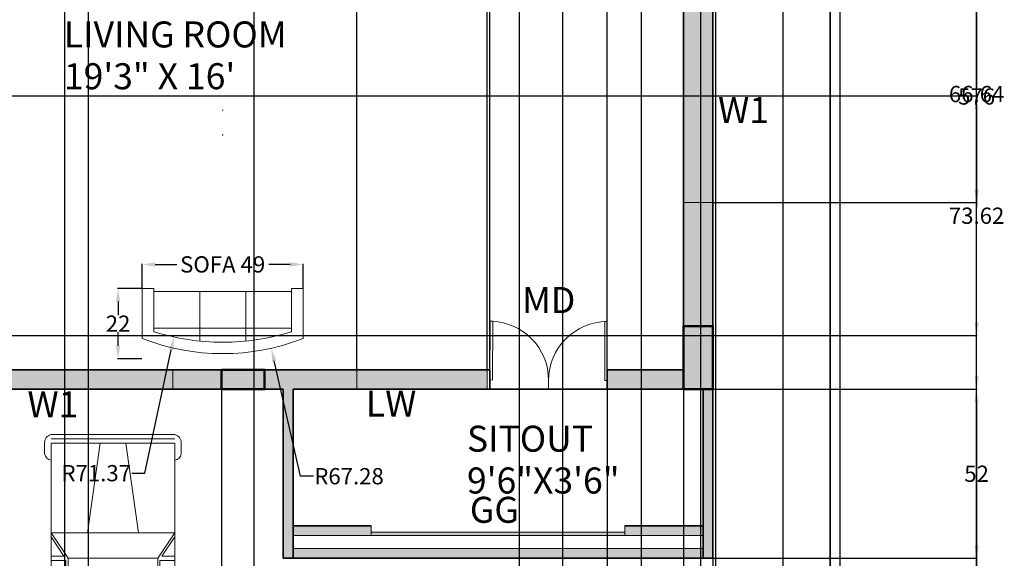
# Model space of a CAD drawing. Units: inches. Extents: x 460 to 1030, y -658 to 271.
# Tile 6 of 10: x 728 to 1030, y -340 to -174. Entities that reach past the tile are written whole.
import ezdxf

# ---------------------------------------------------------------- set-up
doc = ezdxf.new("R2010")
doc.units = ezdxf.units.IN
doc.header["$MEASUREMENT"] = 0
for name, color, linetype, lineweight in [('A-ANNO-DIMS', 2, 'Continuous', 18), ('A-ANNO-TEXT', 7, 'Continuous', 18), ('A-AREA-IDEN', 7, 'Continuous', 25), ('A-COLS', 7, 'Continuous', 50), ('A-DOOR', 3, 'Continuous', 20), ('A-FLOR-STRS', 7, 'Continuous', 18), ('A-FURN', 8, 'Continuous', 18), ('A-GLAZ', 4, 'Continuous', 20), ('A-GLAZ-PATT', 4, 'Continuous', 13), ('A-WALL', 7, 'Continuous', 35), ('A-WALL-PATT', 5, 'Continuous', 13), ('C-PROP', 7, 'Continuous', 25), ('C-SITE-VEHI', 8, 'Continuous', 13)]:
    doc.layers.add(name, color=color, linetype=linetype, lineweight=lineweight)
doc.layers.add('A-COLS-PATT', color=7, linetype='Continuous', lineweight=13, true_color=0xffffff)
doc.styles.get("Standard").update_dxf_attribs({"font": 'arial.ttf'})
doc.dimstyles.get("Standard").update_dxf_attribs({"dimtxt": 5, "dimasz": 4, "dimexe": 0.18, "dimexo": 0.0625, "dimgap": 0.09, "dimtad": 0, "dimtih": 1, "dimtoh": 1, "dimdec": 1, "dimzin": 0, "dimdsep": 46, "dimlunit": 4, "dimtxsty": 'Standard', "dimcen": 0.09, "dimadec": 0, "dimazin": 0, "dimtfac": 1, "dimtdec": 1, "dimtofl": 0, "dimtmove": 0, "dimatfit": 3, "dimfxl": 1, "dimtolj": 1, "dimtzin": 0, "dimarcsym": 0})

# ---------------------------------------------------------------- blocks, each defined once
blk = doc.blocks.new('*U2')
for p, q in [((0, 0), (0, -6)), ((40, 0), (40, -6))]:
    blk.add_line(p, q)
blk.add_lwpolyline([(0, 0), (0, 40), (1.75, 40), (1.75, 0)], close=True)
blk.add_arc((0, 0), 40, 0, 90)
blk = doc.blocks.new('Sofa - Roundback 7 ft.')
for p, q in [((-12.00002, -32.4421), (-12.00003, -6.5971)), ((11.99997, -32.4421), (11.99998, -6.5971)), ((-36.000027, -34), (-36.000027, -11.4696)), ((-35.999844, -13.3819), (35.9998, -13.3819)), ((35.99998, -34), (35.99998, -11.4696)), ((-36.000027, -32.4421), (35.99998, -32.4421))]:
    blk.add_line(p, q)
for points in [[(-36.000027, -34), (-42.000027, -34), (-42.000027, -8)], [(41.99998, -8), (41.99998, -34), (35.99998, -34)]]:
    blk.add_lwpolyline(points)
for centre, radius, start, end in [((0, -114.25), 114.25, 68.43141, 111.5686), ((-0.00001, -127.1968), 121.1968, 72.72033, 107.2797)]:
    blk.add_arc(centre, radius, start, end)
blk = doc.blocks.new('*U14')
for p, q in [((3, -10), (3, 974)), ((70, -10), (70, 973)), ((138, 1075), (308, 1075)), ((138, 973), (410, 973)), ((138, -10), (138, 971)), ((410, 973), (4581, 973)), ((1563, -10), (1563, 973)), ((1563, 973), (1969, 702)), ((1630, 973), (1936, 769)), ((1936, 769), (1936, 973)), ((2003, 973), (2003, 736)), ((2716, 736), (2716, 973)), ((2783, 702), (2783, 973)), ((2851, 973), (2851, 736)), ((3563, 736), (3563, 973)), ((3597, 702), (3801, 973)), ((3801, -10), (3801, 973)), ((4818, 973), (4547, 973)), ((4818, 1075), (4649, 1075)), ((4818, -10), (4818, 971)), ((4886, -10), (4886, 973)), ((4954, -10), (4954, 974)), ((1969, 702), (3597, 702)), ((1969, -10), (1969, 702)), ((2003, 736), (2716, 736)), ((2851, 736), (3563, 736)), ((3597, -10), (3597, 702)), ((138, 193), (1563, 396)), ((3, -11), (3, -995)), ((70, -10), (70, -994)), ((138, -11), (138, -992)), ((1563, -10), (1563, -994)), ((1969, -10), (1969, -723)), ((3597, -10), (3597, -723)), ((3801, -10), (3801, -994)), ((4818, -11), (4818, -992)), ((4886, -10), (4886, -994)), ((4954, -11), (4954, -995)), ((138, -214), (1563, -417)), ((1563, -994), (1969, -723)), ((1969, -723), (3597, -723)), ((2003, -994), (2003, -757)), ((2003, -757), (2716, -757)), ((2716, -757), (2716, -994)), ((2783, -723), (2783, -994)), ((2851, -757), (3563, -757)), ((2851, -994), (2851, -757)), ((3563, -757), (3563, -994)), ((3597, -723), (3801, -994)), ((1630, -994), (1936, -790)), ((1936, -790), (1936, -994)), ((138, -994), (410, -994)), ((138, -1096), (308, -1096)), ((410, -994), (4581, -994)), ((4818, -994), (4547, -994)), ((4818, -1096), (4649, -1096))]:
    blk.add_line(p, q)
for centre, radius, start, end in [((128, 946), 129, 85.6455, 168.0943), ((291, 956), 120, 8.1301, 81.87), ((4665, 956), 120, 98.13, 171.8699), ((4828, 946), 129, 11.9057, 94.3545), ((128, -967), 129, 191.9057, 274.3545), ((291, -977), 120, 278.13, 351.8699), ((4665, -977), 120, 188.1301, 261.87), ((4828, -967), 129, 265.6455, 348.0943)]:
    blk.add_arc(centre, radius, start, end)
blk = doc.blocks.new('*D37')
at = {"layer": 'A-ANNO-DIMS', "color": 0, "lineweight": -2, "transparency": 16777216}
for p, q in [((765.43, -256.72), (765.43, -249.18)), ((769.43, -249.36), (776.02, -249.36)), ((810.89, -249.36), (804.3, -249.36)), ((814.89, -256.72), (814.89, -249.18))]:
    blk.add_line(p, q, dxfattribs=at)
at = {"layer": 'A-ANNO-DIMS', "color": 0, "transparency": 16777216}
for points in [[(769.43, -248.7), (769.43, -250.03), (765.43, -249.36)], [(810.89, -248.7), (810.89, -250.03), (814.89, -249.36)]]:
    blk.add_solid(points, dxfattribs=at)
at = {"layer": 'Defpoints', "color": 0, "transparency": 16777216}
for p in [(765.43, -249.36), (765.43, -256.78), (814.89, -256.78)]:
    blk.add_point(p, dxfattribs=at)
at = {"layer": 'A-ANNO-DIMS', "color": 0, "transparency": 16777216, "insert": (790.16, -249.36), "char_height": 5, "attachment_point": 5}
blk.add_mtext('\\A1;SOFA 49', dxfattribs=at)
blk = doc.blocks.new('*D38')
at = {"layer": 'A-ANNO-DIMS', "color": 0, "lineweight": -2, "transparency": 16777216}
for p, q in [((765.36, -256.78), (757.83, -256.78)), ((758.01, -260.78), (758.01, -264.98)), ((758.01, -274.37), (758.01, -270.18)), ((765.36, -278.37), (757.83, -278.37))]:
    blk.add_line(p, q, dxfattribs=at)
at = {"layer": 'A-ANNO-DIMS', "color": 0, "transparency": 16777216}
for points in [[(757.34, -260.78), (758.67, -260.78), (758.01, -256.78)], [(757.34, -274.37), (758.67, -274.37), (758.01, -278.37)]]:
    blk.add_solid(points, dxfattribs=at)
at = {"layer": 'Defpoints', "color": 0, "transparency": 16777216}
for p in [(765.43, -256.78), (758.01, -278.37), (765.43, -278.37)]:
    blk.add_point(p, dxfattribs=at)
at = {"layer": 'A-ANNO-DIMS', "color": 0, "transparency": 16777216, "insert": (758.01, -267.58), "char_height": 5, "attachment_point": 5}
blk.add_mtext('\\A1;22', dxfattribs=at)
blk = doc.blocks.new('*D41')
at = {"layer": 'A-ANNO-DIMS', "color": 0, "lineweight": -2, "transparency": 16777216}
for p, q in [((979.86, 129.27), (1022.03, 129.27)), ((1021.85, 125.27), (1021.85, -76.63)), ((1021.85, -283.73), (1021.85, -81.83)), ((940.86, -287.73), (1022.03, -287.73))]:
    blk.add_line(p, q, dxfattribs=at)
at = {"layer": 'A-ANNO-DIMS', "color": 0, "transparency": 16777216}
for points in [[(1021.18, 125.27), (1022.51, 125.27), (1021.85, 129.27)], [(1021.18, -283.73), (1022.51, -283.73), (1021.85, -287.73)]]:
    blk.add_solid(points, dxfattribs=at)
at = {"layer": 'Defpoints', "color": 0, "transparency": 16777216}
for p in [(979.8, 129.27), (1021.85, 129.27), (940.8, -287.73)]:
    blk.add_point(p, dxfattribs=at)
at = {"layer": 'A-ANNO-DIMS', "color": 0, "transparency": 16777216, "insert": (1021.85, -79.23), "char_height": 5, "attachment_point": 5}
blk.add_mtext('\\A1;417', dxfattribs=at)
blk = doc.blocks.new('*D42')
at = {"layer": 'A-ANNO-DIMS', "color": 0, "lineweight": -2, "transparency": 16777216}
for p, q in [((940.86, -287.73), (1022.03, -287.73)), ((1021.85, -291.73), (1021.85, -447.08)), ((1021.85, -607.73), (1021.85, -452.37)), ((979.86, -611.73), (1022.03, -611.73))]:
    blk.add_line(p, q, dxfattribs=at)
at = {"layer": 'A-ANNO-DIMS', "color": 0, "transparency": 16777216}
for points in [[(1021.18, -291.73), (1022.51, -291.73), (1021.85, -287.73)], [(1021.18, -607.73), (1022.51, -607.73), (1021.85, -611.73)]]:
    blk.add_solid(points, dxfattribs=at)
at = {"layer": 'Defpoints', "color": 0, "transparency": 16777216}
for p in [(940.8, -287.73), (1021.85, -287.73), (979.8, -611.73)]:
    blk.add_point(p, dxfattribs=at)
at = {"layer": 'A-ANNO-DIMS', "color": 0, "transparency": 16777216, "insert": (1021.85, -449.73), "char_height": 5, "attachment_point": 5}
blk.add_mtext('\\A1;324', dxfattribs=at)
blk = doc.blocks.new('*D44')
at = {"layer": 'A-ANNO-DIMS', "color": 0, "lineweight": -2, "transparency": 16777216}
for p, q in [((940.86, 90.27), (1022.03, 90.27)), ((1021.85, 86.27), (1021.85, -195.08)), ((1021.85, -481.73), (1021.85, -200.37)), ((979.86, -485.73), (1022.03, -485.73))]:
    blk.add_line(p, q, dxfattribs=at)
at = {"layer": 'A-ANNO-DIMS', "color": 0, "transparency": 16777216}
for points in [[(1021.18, 86.27), (1022.51, 86.27), (1021.85, 90.27)], [(1021.18, -481.73), (1022.51, -481.73), (1021.85, -485.73)]]:
    blk.add_solid(points, dxfattribs=at)
at = {"layer": 'Defpoints', "color": 0, "transparency": 16777216}
for p in [(940.8, 90.27), (979.8, -485.73), (1021.85, -485.73)]:
    blk.add_point(p, dxfattribs=at)
at = {"layer": 'A-ANNO-DIMS', "color": 0, "transparency": 16777216, "insert": (1021.85, -197.73), "char_height": 5, "attachment_point": 5}
blk.add_mtext('\\A1;576', dxfattribs=at)
blk = doc.blocks.new('*D45')
at = {"layer": 'A-ANNO-DIMS', "color": 0, "lineweight": -2, "transparency": 16777216}
for p, q in [((976.8, 126.21), (976.8, -654.61)), ((940.8, 90.21), (940.8, -654.61)), ((944.8, -654.43), (955.13, -654.43)), ((972.8, -654.43), (962.46, -654.43))]:
    blk.add_line(p, q, dxfattribs=at)
at = {"layer": 'A-ANNO-DIMS', "color": 0, "transparency": 16777216}
for points in [[(944.8, -653.77), (944.8, -655.1), (940.8, -654.43)], [(972.8, -653.77), (972.8, -655.1), (976.8, -654.43)]]:
    blk.add_solid(points, dxfattribs=at)
at = {"layer": 'Defpoints', "color": 0, "transparency": 16777216}
for p in [(976.8, 126.27), (940.8, 90.27), (976.8, -654.43)]:
    blk.add_point(p, dxfattribs=at)
at = {"layer": 'A-ANNO-DIMS', "color": 0, "transparency": 16777216, "insert": (958.8, -654.43), "char_height": 5, "attachment_point": 5}
blk.add_mtext('\\A1;36', dxfattribs=at)
blk = doc.blocks.new('*D46')
at = {"layer": 'A-ANNO-DIMS', "color": 0, "lineweight": -2, "transparency": 16777216}
for p, q in [((936.98, 127.21), (936.98, -654.61)), ((962.32, 127.21), (962.32, -654.61)), ((932.98, -654.43), (928.98, -654.43)), ((966.32, -654.43), (970.32, -654.43))]:
    blk.add_line(p, q, dxfattribs=at)
at = {"layer": 'A-ANNO-DIMS', "color": 0, "transparency": 16777216}
for points in [[(932.98, -653.77), (932.98, -655.1), (936.98, -654.43)], [(966.32, -653.77), (966.32, -655.1), (962.32, -654.43)]]:
    blk.add_solid(points, dxfattribs=at)
at = {"layer": 'Defpoints', "color": 0, "transparency": 16777216}
for p in [(936.98, 127.27), (962.32, 127.27), (962.32, -654.43)]:
    blk.add_point(p, dxfattribs=at)
at = {"layer": 'A-ANNO-DIMS', "color": 0, "transparency": 16777216, "insert": (949.65, -654.43), "char_height": 5, "attachment_point": 5}
blk.add_mtext('\\A1;25.346', dxfattribs=at)
blk = doc.blocks.new('*D47')
at = {"layer": 'A-ANNO-DIMS', "color": 0, "lineweight": -2, "transparency": 16777216}
for p, q in [((962.32, 129.21), (962.32, -654.61)), ((979.8, 129.21), (979.8, -654.61)), ((966.32, -654.43), (975.8, -654.43)), ((979.8, -654.43), (983.8, -654.43))]:
    blk.add_line(p, q, dxfattribs=at)
at = {"layer": 'A-ANNO-DIMS', "color": 0, "transparency": 16777216}
for points in [[(966.32, -653.77), (966.32, -655.1), (962.32, -654.43)], [(975.8, -653.77), (975.8, -655.1), (979.8, -654.43)]]:
    blk.add_solid(points, dxfattribs=at)
at = {"layer": 'Defpoints', "color": 0, "transparency": 16777216}
for p in [(962.32, 129.27), (979.8, 129.27), (979.8, -654.43)]:
    blk.add_point(p, dxfattribs=at)
at = {"layer": 'A-ANNO-DIMS', "color": 0, "transparency": 16777216, "insert": (994.02, -654.43), "char_height": 5, "attachment_point": 5}
blk.add_mtext('\\A1;17.474', dxfattribs=at)
blk = doc.blocks.new('*D48')
at = {"layer": 'A-ANNO-DIMS', "color": 0, "lineweight": -2, "transparency": 16777216}
for p, q in [((799.88, -611.66), (799.88, 267.89)), ((803.88, 267.71), (860.58, 267.71)), ((937.7, 267.71), (881, 267.71)), ((941.7, -611.66), (941.7, 267.89))]:
    blk.add_line(p, q, dxfattribs=at)
at = {"layer": 'A-ANNO-DIMS', "color": 0, "transparency": 16777216}
for points in [[(803.88, 268.38), (803.88, 267.04), (799.88, 267.71)], [(937.7, 268.38), (937.7, 267.04), (941.7, 267.71)]]:
    blk.add_solid(points, dxfattribs=at)
at = {"layer": 'Defpoints', "color": 0, "transparency": 16777216}
for p in [(941.7, 267.71), (799.88, -611.73), (941.7, -611.73)]:
    blk.add_point(p, dxfattribs=at)
at = {"layer": 'A-ANNO-DIMS', "color": 0, "transparency": 16777216, "insert": (870.79, 267.71), "char_height": 5, "attachment_point": 5}
blk.add_mtext('\\A1;141.82', dxfattribs=at)
blk = doc.blocks.new('*D49')
at = {"layer": 'A-ANNO-DIMS', "color": 0, "lineweight": -2, "transparency": 16777216}
for p, q in [((941.7, -608.66), (941.7, 267.89)), ((945.7, 267.71), (953.15, 267.71)), ((972.8, 267.71), (965.35, 267.71)), ((976.8, -608.66), (976.8, 267.89))]:
    blk.add_line(p, q, dxfattribs=at)
at = {"layer": 'A-ANNO-DIMS', "color": 0, "transparency": 16777216}
for points in [[(945.7, 268.38), (945.7, 267.04), (941.7, 267.71)], [(972.8, 268.38), (972.8, 267.04), (976.8, 267.71)]]:
    blk.add_solid(points, dxfattribs=at)
at = {"layer": 'Defpoints', "color": 0, "transparency": 16777216}
for p in [(976.8, 267.71), (941.7, -608.73), (976.8, -608.73)]:
    blk.add_point(p, dxfattribs=at)
at = {"layer": 'A-ANNO-DIMS', "color": 0, "transparency": 16777216, "insert": (959.25, 267.71), "char_height": 5, "attachment_point": 5}
blk.add_mtext('\\A1;35.1', dxfattribs=at)
blk = doc.blocks.new('*D52')
at = {"layer": 'A-ANNO-DIMS', "color": 0, "lineweight": -2, "transparency": 16777216}
for p, q in [((872.3, -281.66), (872.3, 267.89)), ((876.3, 267.71), (879.84, 267.71)), ((904.35, 267.71), (900.81, 267.71)), ((908.35, -281.66), (908.35, 267.89))]:
    blk.add_line(p, q, dxfattribs=at)
at = {"layer": 'A-ANNO-DIMS', "color": 0, "transparency": 16777216}
for points in [[(876.3, 268.38), (876.3, 267.04), (872.3, 267.71)], [(904.35, 268.38), (904.35, 267.04), (908.35, 267.71)]]:
    blk.add_solid(points, dxfattribs=at)
at = {"layer": 'Defpoints', "color": 0, "transparency": 16777216}
for p in [(908.35, 267.71), (872.3, -281.73), (908.35, -281.73)]:
    blk.add_point(p, dxfattribs=at)
at = {"layer": 'A-ANNO-DIMS', "color": 0, "transparency": 16777216, "insert": (890.32, 267.71), "char_height": 5, "attachment_point": 5}
blk.add_mtext('\\A1;36.045', dxfattribs=at)
blk = doc.blocks.new('*D53')
at = {"layer": 'A-ANNO-DIMS', "color": 0, "lineweight": -2, "transparency": 16777216}
for p, q in [((908.35, -281.79), (908.35, -654.61)), ((931.8, -281.79), (931.8, -654.61)), ((904.35, -654.43), (900.35, -654.43)), ((935.8, -654.43), (939.8, -654.43))]:
    blk.add_line(p, q, dxfattribs=at)
at = {"layer": 'A-ANNO-DIMS', "color": 0, "transparency": 16777216}
for points in [[(904.35, -653.77), (904.35, -655.1), (908.35, -654.43)], [(935.8, -653.77), (935.8, -655.1), (931.8, -654.43)]]:
    blk.add_solid(points, dxfattribs=at)
at = {"layer": 'Defpoints', "color": 0, "transparency": 16777216}
for p in [(908.35, -281.73), (931.8, -281.73), (931.8, -654.43)]:
    blk.add_point(p, dxfattribs=at)
at = {"layer": 'A-ANNO-DIMS', "color": 0, "transparency": 16777216, "insert": (920.07, -654.43), "char_height": 5, "attachment_point": 5}
blk.add_mtext('\\A1;23.45', dxfattribs=at)
blk = doc.blocks.new('*D54')
at = {"layer": 'A-ANNO-DIMS', "color": 0, "lineweight": -2, "transparency": 16777216}
for p, q in [((894.61, -141.78), (894.61, -654.61)), ((931.8, -141.78), (931.8, -654.61)), ((898.61, -654.43), (904.68, -654.43)), ((927.8, -654.43), (921.73, -654.43))]:
    blk.add_line(p, q, dxfattribs=at)
at = {"layer": 'A-ANNO-DIMS', "color": 0, "transparency": 16777216}
for points in [[(898.61, -653.77), (898.61, -655.1), (894.61, -654.43)], [(927.8, -653.77), (927.8, -655.1), (931.8, -654.43)]]:
    blk.add_solid(points, dxfattribs=at)
at = {"layer": 'Defpoints', "color": 0, "transparency": 16777216}
for p in [(894.61, -141.72), (931.8, -141.72), (931.8, -654.43)]:
    blk.add_point(p, dxfattribs=at)
at = {"layer": 'A-ANNO-DIMS', "color": 0, "transparency": 16777216, "insert": (913.2, -654.43), "char_height": 5, "attachment_point": 5}
blk.add_mtext('\\A1;37.18', dxfattribs=at)
blk = doc.blocks.new('*D57')
at = {"layer": 'A-ANNO-DIMS', "color": 0, "lineweight": -2, "transparency": 16777216}
for p, q in [((717.53, -38.79), (717.53, -654.61)), ((741.59, -38.79), (741.59, -654.61)), ((713.53, -654.43), (709.53, -654.43)), ((745.59, -654.43), (749.59, -654.43))]:
    blk.add_line(p, q, dxfattribs=at)
at = {"layer": 'A-ANNO-DIMS', "color": 0, "transparency": 16777216}
for points in [[(713.53, -653.77), (713.53, -655.1), (717.53, -654.43)], [(745.59, -653.77), (745.59, -655.1), (741.59, -654.43)]]:
    blk.add_solid(points, dxfattribs=at)
at = {"layer": 'Defpoints', "color": 0, "transparency": 16777216}
for p in [(717.53, -38.73), (741.59, -38.73), (741.59, -654.43)]:
    blk.add_point(p, dxfattribs=at)
at = {"layer": 'A-ANNO-DIMS', "color": 0, "transparency": 16777216, "insert": (729.56, -654.43), "char_height": 5, "attachment_point": 5}
blk.add_mtext('\\A1;24.065', dxfattribs=at)
blk = doc.blocks.new('*D60')
at = {"layer": 'A-ANNO-DIMS', "color": 0, "lineweight": -2, "transparency": 16777216}
for p, q in [((940.86, -163.66), (1022.03, -163.66)), ((1021.85, -167.66), (1021.85, -194.33)), ((1021.85, -226.29), (1021.85, -199.62)), ((940.86, -230.29), (1022.03, -230.29))]:
    blk.add_line(p, q, dxfattribs=at)
at = {"layer": 'A-ANNO-DIMS', "color": 0, "transparency": 16777216}
for points in [[(1021.18, -167.66), (1022.51, -167.66), (1021.85, -163.66)], [(1021.18, -226.29), (1022.51, -226.29), (1021.85, -230.29)]]:
    blk.add_solid(points, dxfattribs=at)
at = {"layer": 'Defpoints', "color": 0, "transparency": 16777216}
for p in [(940.8, -163.66), (940.8, -230.29), (1021.85, -230.29)]:
    blk.add_point(p, dxfattribs=at)
at = {"layer": 'A-ANNO-DIMS', "color": 0, "transparency": 16777216, "insert": (1021.85, -196.98), "char_height": 5, "attachment_point": 5}
blk.add_mtext('\\A1;66.64', dxfattribs=at)
blk = doc.blocks.new('*D62')
at = {"layer": 'A-ANNO-DIMS', "color": 0, "lineweight": -2, "transparency": 16777216}
for p, q in [((700.86, -197.58), (1022.03, -197.58)), ((1021.85, -201.58), (1021.85, -231.74)), ((1021.85, -267.2), (1021.85, -237.03)), ((700.86, -271.2), (1022.03, -271.2))]:
    blk.add_line(p, q, dxfattribs=at)
at = {"layer": 'A-ANNO-DIMS', "color": 0, "transparency": 16777216}
for points in [[(1021.18, -201.58), (1022.51, -201.58), (1021.85, -197.58)], [(1021.18, -267.2), (1022.51, -267.2), (1021.85, -271.2)]]:
    blk.add_solid(points, dxfattribs=at)
at = {"layer": 'Defpoints', "color": 0, "transparency": 16777216}
for p in [(700.8, -197.58), (700.8, -271.2), (1021.85, -271.2)]:
    blk.add_point(p, dxfattribs=at)
at = {"layer": 'A-ANNO-DIMS', "color": 0, "transparency": 16777216, "insert": (1021.85, -234.39), "char_height": 5, "attachment_point": 5}
blk.add_mtext('\\A1;73.62', dxfattribs=at)
blk = doc.blocks.new('*D67')
at = {"layer": 'A-ANNO-DIMS', "color": 0, "lineweight": -2, "transparency": 16777216}
for p, q in [((940.86, -287.73), (1022.03, -287.73)), ((1021.85, -291.73), (1021.85, -311.08)), ((1021.85, -335.73), (1021.85, -316.37)), ((940.86, -339.73), (1022.03, -339.73))]:
    blk.add_line(p, q, dxfattribs=at)
at = {"layer": 'A-ANNO-DIMS', "color": 0, "transparency": 16777216}
for points in [[(1021.18, -291.73), (1022.51, -291.73), (1021.85, -287.73)], [(1021.18, -335.73), (1022.51, -335.73), (1021.85, -339.73)]]:
    blk.add_solid(points, dxfattribs=at)
at = {"layer": 'Defpoints', "color": 0, "transparency": 16777216}
for p in [(940.8, -287.73), (1021.85, -287.73), (940.8, -339.73)]:
    blk.add_point(p, dxfattribs=at)
at = {"layer": 'A-ANNO-DIMS', "color": 0, "transparency": 16777216, "insert": (1021.85, -313.73), "char_height": 5, "attachment_point": 5}
blk.add_mtext('\\A1;52', dxfattribs=at)
blk = doc.blocks.new('*D69')
at = {"layer": 'A-ANNO-DIMS', "color": 0, "lineweight": -2, "transparency": 16777216}
for p, q in [((881.27, 90.21), (881.27, -654.61)), ((918.77, 90.21), (918.77, -654.61)), ((885.27, -654.43), (893.42, -654.43)), ((914.77, -654.43), (906.62, -654.43))]:
    blk.add_line(p, q, dxfattribs=at)
at = {"layer": 'A-ANNO-DIMS', "color": 0, "transparency": 16777216}
for points in [[(885.27, -653.77), (885.27, -655.1), (881.27, -654.43)], [(914.77, -653.77), (914.77, -655.1), (918.77, -654.43)]]:
    blk.add_solid(points, dxfattribs=at)
at = {"layer": 'Defpoints', "color": 0, "transparency": 16777216}
for p in [(881.27, 90.27), (918.77, 90.27), (918.77, -654.43)]:
    blk.add_point(p, dxfattribs=at)
at = {"layer": 'A-ANNO-DIMS', "color": 0, "transparency": 16777216, "insert": (900.02, -654.43), "char_height": 5, "attachment_point": 5}
blk.add_mtext('\\A1;37.5', dxfattribs=at)
blk = doc.blocks.new('*D70')
at = {"layer": 'A-ANNO-DIMS', "color": 0, "lineweight": -2, "transparency": 16777216}
for p, q in [((716.71, -287.79), (716.71, -654.61)), ((789.82, -287.79), (789.82, -654.61)), ((720.71, -654.43), (744.79, -654.43)), ((785.82, -654.43), (761.75, -654.43))]:
    blk.add_line(p, q, dxfattribs=at)
at = {"layer": 'A-ANNO-DIMS', "color": 0, "transparency": 16777216}
for points in [[(720.71, -653.77), (720.71, -655.1), (716.71, -654.43)], [(785.82, -653.77), (785.82, -655.1), (789.82, -654.43)]]:
    blk.add_solid(points, dxfattribs=at)
at = {"layer": 'Defpoints', "color": 0, "transparency": 16777216}
for p in [(716.71, -287.73), (789.82, -287.73), (789.82, -654.43)]:
    blk.add_point(p, dxfattribs=at)
at = {"layer": 'A-ANNO-DIMS', "color": 0, "transparency": 16777216, "insert": (753.27, -654.43), "char_height": 5, "attachment_point": 5}
blk.add_mtext('\\A1;73.12', dxfattribs=at)
blk = doc.blocks.new('*D71')
at = {"layer": 'A-ANNO-DIMS', "color": 0, "lineweight": -2, "transparency": 16777216}
for p, q in [((831.43, -281.66), (831.43, 267.89)), ((835.43, 267.71), (840.88, 267.71)), ((867.46, 267.71), (862.01, 267.71)), ((871.46, -281.66), (871.46, 267.89))]:
    blk.add_line(p, q, dxfattribs=at)
at = {"layer": 'A-ANNO-DIMS', "color": 0, "transparency": 16777216}
for points in [[(835.43, 268.38), (835.43, 267.04), (831.43, 267.71)], [(867.46, 268.38), (867.46, 267.04), (871.46, 267.71)]]:
    blk.add_solid(points, dxfattribs=at)
at = {"layer": 'Defpoints', "color": 0, "transparency": 16777216}
for p in [(871.46, 267.71), (831.43, -281.73), (871.46, -281.73)]:
    blk.add_point(p, dxfattribs=at)
at = {"layer": 'A-ANNO-DIMS', "color": 0, "transparency": 16777216, "insert": (851.44, 267.71), "char_height": 5, "attachment_point": 5}
blk.add_mtext('\\A1;40.026', dxfattribs=at)
blk = doc.blocks.new('*D72')
at = {"layer": 'A-ANNO-DIMS', "color": 0, "lineweight": -2, "transparency": 16777216}
for p, q in [((715.8, 68.25), (715.8, -654.61)), ((748.8, 57.75), (748.8, -654.61)), ((719.8, -654.43), (728.63, -654.43)), ((744.8, -654.43), (735.97, -654.43))]:
    blk.add_line(p, q, dxfattribs=at)
at = {"layer": 'A-ANNO-DIMS', "color": 0, "transparency": 16777216}
for points in [[(719.8, -653.77), (719.8, -655.1), (715.8, -654.43)], [(744.8, -653.77), (744.8, -655.1), (748.8, -654.43)]]:
    blk.add_solid(points, dxfattribs=at)
at = {"layer": 'Defpoints', "color": 0, "transparency": 16777216}
for p in [(715.8, 68.31), (748.8, 57.81), (748.8, -654.43)]:
    blk.add_point(p, dxfattribs=at)
at = {"layer": 'A-ANNO-DIMS', "color": 0, "transparency": 16777216, "insert": (732.3, -654.43), "char_height": 5, "attachment_point": 5}
blk.add_mtext('\\A1;33', dxfattribs=at)
blk = doc.blocks.new('*D78')
at = {"layer": 'A-ANNO-DIMS', "color": 0, "lineweight": -2, "transparency": 16777216}
for p, q in [((790.07, -201.9), (790.25, -201.9)), ((790.16, -201.99), (790.16, -201.81)), ((766.22, -313.55), (774.36, -275.6)), ((762.22, -313.55), (766.22, -313.55))]:
    blk.add_line(p, q, dxfattribs=at)
at = {"layer": 'A-ANNO-DIMS', "color": 0, "transparency": 16777216}
blk.add_solid([(773.71, -275.46), (775.01, -275.74), (775.2, -271.68)], dxfattribs=at)
at = {"layer": 'Defpoints', "color": 0, "transparency": 16777216}
for p in [(790.16, -201.9), (775.2, -271.68)]:
    blk.add_point(p, dxfattribs=at)
at = {"layer": 'A-ANNO-DIMS', "color": 0, "transparency": 16777216, "insert": (751.3, -313.55), "char_height": 5, "attachment_point": 5}
blk.add_mtext('\\A1;R71.37', dxfattribs=at)
blk = doc.blocks.new('*D79')
at = {"layer": 'A-ANNO-DIMS', "color": 0, "lineweight": -2, "transparency": 16777216}
for p, q in [((790.07, -209.53), (790.25, -209.53)), ((790.16, -209.62), (790.16, -209.44)), ((814.07, -314.48), (805.99, -279.02)), ((818.07, -314.48), (814.07, -314.48))]:
    blk.add_line(p, q, dxfattribs=at)
at = {"layer": 'A-ANNO-DIMS', "color": 0, "transparency": 16777216}
blk.add_solid([(806.64, -278.88), (805.34, -279.17), (805.1, -275.12)], dxfattribs=at)
at = {"layer": 'Defpoints', "color": 0, "transparency": 16777216}
for p in [(790.16, -209.53), (805.1, -275.12)]:
    blk.add_point(p, dxfattribs=at)
at = {"layer": 'A-ANNO-DIMS', "color": 0, "transparency": 16777216, "insert": (828.99, -314.48), "char_height": 5, "attachment_point": 5}
blk.add_mtext('\\A1;R67.28', dxfattribs=at)

msp = doc.modelspace()

# ---------------------------------------------------------------- hatches: boundary and pattern name
at = {"layer": 'A-COLS-PATT'}
h = msp.add_hatch(color=256, dxfattribs=at)
h.dxf.hatch_style = 1
h.paths.add_polyline_path([(571.7961, 90.2738), (562.7961, 90.2738), (562.7961, 71.6966), (571.7961, 71.6966)])
h.paths.add_polyline_path([(700.7961, 90.2738), (691.7961, 90.2738), (691.7961, 71.6966), (700.7961, 71.6966)])
h.paths.add_polyline_path([(811.7961, 90.2738), (802.7961, 90.2738), (802.7961, 71.6966), (811.7961, 71.6966)])
h.paths.add_polyline_path([(940.7961, 90.2738), (931.7961, 90.2738), (931.7961, 71.6966), (940.7961, 71.6966)])
h.paths.add_polyline_path([(940.7961, -101.149), (931.7961, -101.149), (931.7961, -119.7262), (940.7961, -119.7262)])
h.paths.add_polyline_path([(940.7961, -268.3723), (931.7961, -268.3723), (931.7961, -287.7262), (940.7961, -287.7262)])
h.paths.add_polyline_path([(803.0275, -281.7262), (789.8237, -281.7262), (789.8237, -287.7262), (803.0275, -287.7262)])
h.paths.add_polyline_path([(700.7961, -303.809), (691.7961, -303.809), (691.7961, -323.8443), (700.7961, -323.8443)])
h.paths.add_polyline_path([(571.7961, -303.809), (562.7961, -303.809), (562.7961, -323.8443), (571.7961, -323.8443)])
h.paths.add_polyline_path([(571.7961, -413.1453), (562.7961, -413.1453), (562.7961, -432.4659), (571.7961, -432.4659)])
h.paths.add_polyline_path([(571.7961, -101.149), (562.7961, -101.149), (562.7961, -119.7262), (571.7961, -119.7262)])
h.paths.add_polyline_path([(700.7961, -101.0985), (691.7961, -101.0985), (691.7961, -119.7262), (700.7961, -119.7262)])
h.paths.add_polyline_path([(811.7961, -101.149), (802.7961, -101.149), (802.7961, -119.7262), (811.7961, -119.7262)])
at = {"layer": 'A-GLAZ-PATT'}
h = msp.add_hatch(color=256, dxfattribs=at)
h.dxf.hatch_style = 1
h.paths.add_polyline_path([(571.7961, -343.9041), (562.7961, -343.9041), (562.7961, -384.3969), (571.7961, -384.3969)])
h.paths.add_polyline_path([(571.7961, -143.2895), (562.7961, -143.2895), (562.7961, -168.3798), (571.7961, -168.3798)])
h.paths.add_polyline_path([(571.7961, -49.2966), (562.7961, -49.2966), (562.7961, -90.3192), (571.7961, -90.3192)])
h.paths.add_polyline_path([(666.4584, 90.2738), (634.2742, 90.2738), (634.2742, 81.2738), (666.4584, 81.2738)])
h.paths.add_polyline_path([(742.1779, 90.2738), (713.201, 90.2738), (713.201, 81.2738), (742.1779, 81.2738)])
h.paths.add_polyline_path([(797.2395, 90.2738), (768.2626, 90.2738), (768.2626, 81.2738), (797.2395, 81.2738)])
h.paths.add_polyline_path([(918.7723, 90.2738), (881.2728, 90.2738), (881.2728, 81.2738), (918.7723, 81.2738)])
h.paths.add_polyline_path([(940.7961, -60.0042), (931.7961, -60.0042), (931.7961, -95.7262), (940.7961, -95.7262)])
h.paths.add_polyline_path([(940.7961, -163.6558), (931.7961, -163.6558), (931.7961, -230.2946), (940.7961, -230.2946)])
h.paths.add_polyline_path([(913.7961, -331.7262), (835.7961, -331.7262), (835.7961, -332.7262), (913.7961, -332.7262)])
h.paths.add_polyline_path([(871.4559, -281.7262), (831.4302, -281.7262), (831.4302, -287.7262), (871.4559, -287.7262)])
h.paths.add_polyline_path([(774.8576, -281.7262), (716.7073, -281.7262), (716.7073, -287.7262), (774.8576, -287.7262)])
at = {"layer": 'A-WALL-PATT'}
h = msp.add_hatch(color=256, dxfattribs=at)
h.dxf.hatch_style = 1
h.paths.add_polyline_path([(634.2742, 90.2738), (571.7961, 90.2738), (571.7961, 81.2738), (634.2742, 81.2738)])
h.paths.add_polyline_path([(691.7961, 90.2738), (666.4584, 90.2738), (666.4584, 81.2738), (691.7961, 81.2738)])
h.paths.add_polyline_path([(713.201, 90.2738), (700.7961, 90.2738), (700.7961, 81.2738), (713.201, 81.2738)])
h.paths.add_polyline_path([(748.7961, 90.2738), (742.1779, 90.2738), (742.1779, 81.2738), (748.7961, 81.2738)])
h.paths.add_polyline_path([(768.2626, 90.2738), (754.7961, 90.2738), (754.7961, 81.2738), (768.2626, 81.2738)])
h.paths.add_polyline_path([(802.7961, 90.2738), (797.2395, 90.2738), (797.2395, 81.2738), (802.7961, 81.2738)])
h.paths.add_polyline_path([(881.2728, 90.2738), (811.7961, 90.2738), (811.7961, 81.2738), (881.2728, 81.2738)])
h.paths.add_polyline_path([(931.7961, 90.2738), (918.7723, 90.2738), (918.7723, 81.2738), (931.7961, 81.2738)])
h.paths.add_polyline_path([(940.7961, 71.6966), (931.7961, 71.6966), (931.7961, -60.0042), (940.7961, -60.0042)])
h.paths.add_polyline_path([(940.7961, -95.7262), (931.7961, -95.7262), (931.7961, -101.149), (940.7961, -101.149)])
h.paths.add_polyline_path([(931.7961, -110.7262), (894.6225, -110.7262), (894.6225, -119.7262), (931.7961, -119.7262)])
h.paths.add_polyline_path([(858.6225, -110.7262), (811.7961, -110.7262), (811.7961, -119.7262), (858.6225, -119.7262)])
h.paths.add_polyline_path([(940.7961, -119.7262), (931.7961, -119.7262), (931.7961, -141.7212), (931.7961, -163.6558), (940.7961, -163.6558)])
h.paths.add_polyline_path([(940.7961, -230.2946), (931.7961, -230.2946), (931.7961, -268.3723), (940.7961, -268.3723)])
h.paths.add_polyline_path([(931.7961, -281.7262), (908.3452, -281.7262), (908.3452, -285.0181), (908.3452, -287.7262), (931.7961, -287.7262)])
h.paths.add_polyline_path([(831.4302, -281.7262), (803.0275, -281.7262), (803.0275, -287.7262), (808.7961, -287.7262), (808.7961, -339.7262), (811.7961, -339.7262), (811.7961, -287.7262), (831.4302, -287.7262)])
h.paths.add_polyline_path([(789.8237, -281.7262), (774.8576, -281.7262), (774.8576, -287.7262), (789.8237, -287.7262)])
h.paths.add_polyline_path([(716.7073, -281.7262), (700.7961, -281.7262), (700.7961, -271.1977), (691.7961, -271.1977), (691.7961, -281.7262), (682.4735, -281.7262), (682.4735, -287.7262), (691.7961, -287.7262), (691.7961, -303.809), (700.7961, -303.809), (700.7961, -287.7262), (716.7073, -287.7262)])
h.paths.add_polyline_path([(700.7961, -323.8443), (691.7961, -323.8443), (691.7961, -413.1453), (700.7961, -413.1453)])
h.paths.add_polyline_path([(940.7961, -287.7262), (937.7961, -287.7262), (937.7961, -339.7262), (940.7961, -339.7262)])
h.paths.add_polyline_path([(937.7961, -336.7262), (811.7961, -336.7262), (811.7961, -339.7262), (937.7961, -339.7262)])
h.paths.add_polyline_path([(835.7961, -329.7262), (811.7961, -329.7262), (811.7961, -332.7262), (835.7961, -332.7262)])
h.paths.add_polyline_path([(937.7961, -329.7262), (913.7961, -329.7262), (913.7961, -332.7262), (937.7961, -332.7262)])
h.paths.add_polyline_path([(691.7961, -419.7262), (681.4044, -419.7262), (681.4044, -428.7262), (691.7961, -428.7262)])
h.paths.add_polyline_path([(691.7961, -476.7262), (571.7961, -476.7262), (571.7961, -485.7262), (691.7961, -485.7262)])
h.paths.add_polyline_path([(571.7961, -465.0348), (568.223, -465.0348), (562.7961, -465.0348), (562.7961, -476.7262), (571.7961, -476.7262)])
h.paths.add_polyline_path([(571.7961, -432.4659), (562.7961, -432.4659), (562.7961, -441.1912), (571.7961, -441.1912)])
h.paths.add_polyline_path([(571.7961, -384.3969), (562.7961, -384.3969), (562.7961, -413.1453), (571.7961, -413.1453)])
h.paths.add_polyline_path([(571.7961, -323.8443), (562.7961, -323.8443), (562.7961, -343.9041), (571.7961, -343.9041)])
h.paths.add_polyline_path([(571.7961, -287.7262), (646.4735, -287.7262), (646.4735, -281.7262), (571.7961, -281.7262), (571.7961, -258.1542), (571.7961, -233.7262), (566.4164, -233.7262), (562.7961, -233.7262), (562.7961, -303.809), (571.7961, -303.809)])
h.paths.add_polyline_path([(571.7961, -179.7262), (691.7961, -179.7262), (691.7961, -197.5753), (700.7961, -197.5753), (700.7961, -173.7262), (647.7961, -173.7262), (647.7961, -165.5723), (643.7961, -165.5723), (643.7961, -173.7262), (571.7961, -173.7262), (571.7961, -168.3798), (562.7961, -168.3798), (562.7961, -197.7262), (571.7961, -197.7262)])
h.paths.add_polyline_path([(647.7961, -110.7262), (571.7961, -110.7262), (571.7961, -119.7262), (643.7961, -119.7262), (643.7961, -141.5723), (647.7961, -141.5723)])
h.paths.add_polyline_path([(691.7961, -110.7262), (683.7961, -110.7262), (683.7961, -114.3453), (683.7961, -119.7262), (691.7961, -119.7262)])
h.paths.add_polyline_path([(571.7961, -119.7262), (562.7961, -119.7262), (562.7961, -143.2895), (571.7961, -143.2895)])
h.paths.add_polyline_path([(571.7961, -90.3192), (562.7961, -90.3192), (562.7961, -101.149), (571.7961, -101.149)])
h.paths.add_polyline_path([(571.7961, 71.6966), (562.7961, 71.6966), (562.7961, -49.2966), (571.7961, -49.2966)])
h.paths.add_polyline_path([(700.7961, 71.6966), (691.7961, 71.6966), (691.7961, -50.298), (700.7961, -50.298)])
h.paths.add_polyline_path([(754.7961, 81.2738), (748.7961, 81.2738), (748.7961, -38.7262), (741.5908, -38.7262), (741.5908, -39.109), (741.5908, -42.7262), (748.7961, -42.7262), (748.7961, -110.7262), (754.7961, -110.7262), (754.7961, -42.7262), (773.6274, -42.7262), (773.6274, -38.7262), (754.7961, -38.7262)])
h.paths.add_polyline_path([(717.4759, -38.7262), (700.7961, -38.7262), (700.7961, -42.7262), (717.4759, -42.7262)])
h.paths.add_polyline_path([(811.7961, 71.6966), (802.7961, 71.6966), (802.7961, -50.298), (811.7961, -50.298)])
h.paths.add_polyline_path([(811.7961, -86.298), (806.4164, -86.298), (802.7961, -86.298), (802.7961, -101.149), (811.7961, -101.149)])

# ---------------------------------------------------------------- linework, layer by layer
at = {"layer": 'A-COLS'}
for points in [[(940.7961, -287.7262), (931.7961, -287.7262), (931.7961, -268.3723), (940.7961, -268.3723)], [(789.8237, -281.7262), (803.0275, -281.7262), (803.0275, -287.7262), (789.8237, -287.7262)]]:
    msp.add_lwpolyline(points, close=True, dxfattribs=at)
at = {"layer": 'A-DOOR'}
for p, q in [((835.7961, -329.7262), (835.7961, -332.7262)), ((913.7961, -329.7262), (913.7961, -332.7262)), ((913.7961, -331.7262), (835.7961, -331.7262))]:
    msp.add_line(p, q, dxfattribs=at)
at = {"layer": 'A-FLOR-STRS'}
for p, q in [((937.7961, -332.7262), (811.7961, -332.7262)), ((937.7961, -336.7262), (811.7961, -336.7262))]:
    msp.add_line(p, q, dxfattribs=at)
at = {"layer": 'A-GLAZ'}
for points in [[(940.7961, -230.2946), (931.7961, -230.2946), (931.7961, -163.6558), (940.7961, -163.6558)], [(716.7073, -281.7262), (774.8576, -281.7262), (774.8576, -287.7262), (716.7073, -287.7262)], [(831.4302, -281.7262), (871.4559, -281.7262), (871.4559, -287.7262), (831.4302, -287.7262)]]:
    msp.add_lwpolyline(points, close=True, dxfattribs=at)
at = {"layer": 'A-WALL'}
for p, q in [((940.7961, 90.2738), (940.7961, -281.7262)), ((931.7961, 81.2738), (931.7961, -281.7262)), ((872.2999, -281.7262), (700.7961, -281.7262)), ((872.2999, -287.7262), (872.2999, -281.7262)), ((931.7961, -281.7262), (908.3452, -281.7262)), ((908.3452, -287.7262), (908.3452, -281.7262)), ((940.7961, -281.7262), (940.7961, -339.7262)), ((808.7961, -287.7262), (700.7961, -287.7262)), ((808.7961, -287.7262), (808.7961, -339.7262)), ((940.7961, -287.7262), (811.7961, -287.7262)), ((811.7961, -287.7262), (811.7961, -339.7262)), ((937.7961, -287.7262), (937.7961, -339.7262)), ((825.068, -329.7262), (811.7961, -329.7262)), ((835.7961, -329.7262), (811.7961, -329.7262)), ((937.7961, -329.7262), (913.7961, -329.7262)), ((940.7961, -339.7262), (808.7961, -339.7262))]:
    msp.add_line(p, q, dxfattribs=at)
at = {"layer": 'C-PROP'}
for p, q in [((979.7961, 129.2738), (979.7961, -524.7262)), ((976.7961, 126.2738), (976.7961, -466.833))]:
    msp.add_line(p, q, dxfattribs=at)

# ---------------------------------------------------------------- block references
at = {"layer": 'A-DOOR', "xscale": 0.4513494847069392, "yscale": 0.4513494847069392, "zscale": 0.4513494847069392, "rotation": 359.6322076213278}
msp.add_blockref('*U2', (872.255, -284.9023), dxfattribs=at)
at = {"layer": 'A-DOOR', "xscale": -0.451349484706939, "yscale": 0.451349484706939, "zscale": 0.451349484706939}
msp.add_blockref('*U2', (908.3452, -285.0181), dxfattribs=at)
at = {"layer": 'A-FURN', "xscale": 0.5888541577476372, "yscale": 0.5888541577476372, "zscale": 0.5888541577476372, "rotation": 180}
msp.add_blockref('Sofa - Roundback 7 ft.', (790.159, -276.8035), dxfattribs=at)
at = {"layer": 'C-SITE-VEHI', "xscale": 0.0193263137064046, "yscale": 0.0193263137064046, "zscale": 0.0193263137064046, "rotation": 270}
msp.add_blockref('*U14', (756.6242, -301.6472), dxfattribs=at)

# ---------------------------------------------------------------- texts
at = {"layer": 'A-ANNO-TEXT'}
for s, p in [('W1', (942.3967, -205.9109)), ('MD', (882.1652, -264.3395)), ('W1', (730.1562, -296.374)), ('LW', (834.1654, -296.1327)), ('GG', (866.1279, -328.8122))]:
    msp.add_text(s, height=8, dxfattribs=at).set_placement(p)
at = {"layer": 'A-AREA-IDEN'}
for s, p in [('LIVING ROOM', (741.3655, -182.6601)), ('19\'3" X 16\'', (741.3655, -195.5114)), ('SITOUT', (865.2295, -306.9516)), ('9\'6"X3\'6"', (865.2295, -319.8029))]:
    msp.add_text(s, height=8, dxfattribs=at).set_placement(p)

# ---------------------------------------------------------------- dimensions: what is measured, and where the dimension line sits
at = {"layer": 'A-ANNO-DIMS'}
for base, p1, p2, override, picture, middle in [((941.6978, 267.7108), (799.8801, -611.7262), (941.6978, -611.7262), {"dimdec": 2, "dimlfac": 1, "dimrnd": 0, "dimzin": 0, "dimdsep": 46, "dimlunit": 2}, '*D48', (870.7889, 267.7108)), ((871.4559, 267.7108), (831.4302, -281.7262), (871.4559, -281.7262), {"dimdec": 3, "dimlfac": 1, "dimrnd": 0, "dimzin": 0, "dimdsep": 46, "dimlunit": 2}, '*D71', (851.443, 267.7108)), ((908.3452, 267.7108), (872.2999, -281.7262), (908.3452, -281.7262), {"dimdec": 3, "dimlfac": 1, "dimrnd": 0, "dimzin": 0, "dimdsep": 46, "dimlunit": 2}, '*D52', (890.3226, 267.7108)), ((976.7961, 267.7108), (941.6978, -608.7262), (976.7961, -608.7262), {"dimdec": 1, "dimlfac": 1, "dimrnd": 0, "dimzin": 0, "dimdsep": 46, "dimlunit": 2}, '*D49', (959.247, 267.7108)), ((962.3217, -654.4339), (936.9757, 127.2738), (962.3217, 127.2738), {"dimdec": 3, "dimlfac": 1, "dimrnd": 0, "dimzin": 0, "dimdsep": 46, "dimlunit": 2}, '*D46', (949.6487, -654.4339)), ((979.7961, -654.4339), (962.3217, 129.2738), (979.7961, 129.2738), {"dimdec": 3, "dimlfac": 1, "dimrnd": 0, "dimzin": 0, "dimdsep": 46, "dimlunit": 2}, '*D47', (994.0191, -654.4339)), ((976.7961, -654.4339), (940.7961, 90.2738), (976.7961, 126.2738), {"dimdec": 0, "dimlfac": 1, "dimrnd": 0, "dimzin": 0, "dimdsep": 46, "dimlunit": 2}, '*D45', (958.7961, -654.4339)), ((918.7723, -654.4339), (881.2728, 90.2738), (918.7723, 90.2738), {"dimdec": 1, "dimlfac": 1, "dimrnd": 0, "dimzin": 0, "dimdsep": 46, "dimlunit": 2}, '*D69', (900.0226, -654.4339)), ((748.7961, -654.4339), (715.7961, 68.3148), (748.7961, 57.8148), {"dimdec": 0, "dimlfac": 1, "dimrnd": 0, "dimzin": 0, "dimdsep": 46, "dimlunit": 2}, '*D72', (732.2961, -654.4339)), ((741.5908, -654.4339), (717.5258, -38.7262), (741.5908, -38.7262), {"dimdec": 3, "dimlfac": 1, "dimrnd": 0, "dimzin": 0, "dimdsep": 46, "dimlunit": 2}, '*D57', (729.5583, -654.4339)), ((931.7961, -654.4339), (894.6132, -141.7212), (931.7961, -141.7212), {"dimdec": 2, "dimlfac": 1, "dimrnd": 0, "dimzin": 0, "dimdsep": 46, "dimlunit": 2}, '*D54', (913.2047, -654.4339)), ((931.7961, -654.4339), (908.3452, -281.7262), (931.7961, -281.7262), {"dimdec": 2, "dimlfac": 1, "dimrnd": 0, "dimzin": 0, "dimdsep": 46, "dimlunit": 2}, '*D53', (920.0707, -654.4339)), ((789.8237, -654.4339), (716.7073, -287.7262), (789.8237, -287.7262), {"dimdec": 2, "dimlfac": 1, "dimrnd": 0, "dimzin": 0, "dimdsep": 46, "dimlunit": 2}, '*D70', (753.2655, -654.4339))]:
    dim = msp.add_linear_dim(base=base, p1=p1, p2=p2, dimstyle='Standard', override=override, dxfattribs=at)
    dim.commit()
    dim.dimension.update_dxf_attribs({"geometry": picture, "text_midpoint": middle})
for base, p1, p2, angle, override, picture, middle in [((1021.8461, 129.2738), (940.7961, -287.7262), (979.7961, 129.2738), 90, {"dimdec": 0, "dimlfac": 1, "dimrnd": 0, "dimzin": 0, "dimdsep": 46, "dimlunit": 2}, '*D41', (1021.8461, -79.2262)), ((1021.8461, -485.7262), (940.7961, 90.2738), (979.7961, -485.7262), 90, {"dimdec": 0, "dimlfac": 1, "dimrnd": 0, "dimzin": 0, "dimdsep": 46, "dimlunit": 2}, '*D44', (1021.8461, -197.7262)), ((1021.8461, -230.2946), (940.7961, -163.6558), (940.7961, -230.2946), 90, {"dimdec": 2, "dimlfac": 1, "dimrnd": 0, "dimzin": 0, "dimdsep": 46, "dimlunit": 2}, '*D60', (1021.8461, -196.9752)), ((1021.8461, -271.1977), (700.7961, -197.5753), (700.7961, -271.1977), 90, {"dimdec": 2, "dimlfac": 1, "dimrnd": 0, "dimzin": 0, "dimdsep": 46, "dimlunit": 2}, '*D62', (1021.8461, -234.3865)), ((758.0076, -278.3737), (765.4271, -256.7824), (765.4271, -278.3737), 270, {"dimdec": 0, "dimlfac": 1, "dimrnd": 0, "dimzin": 0, "dimdsep": 46, "dimlunit": 2}, '*D38', (758.0076, -267.5781)), ((1021.8461, -287.7262), (979.7961, -611.7262), (940.7961, -287.7262), 90, {"dimdec": 0, "dimlfac": 1, "dimrnd": 0, "dimzin": 0, "dimdsep": 46, "dimlunit": 2}, '*D42', (1021.8461, -449.7262)), ((1021.8461, -287.7262), (940.7961, -339.7262), (940.7961, -287.7262), 90, {"dimdec": 0, "dimlfac": 1, "dimrnd": 0, "dimzin": 0, "dimdsep": 46, "dimlunit": 2}, '*D67', (1021.8461, -313.7262))]:
    dim = msp.add_linear_dim(base=base, p1=p1, p2=p2, angle=angle, dimstyle='Standard', override=override, dxfattribs=at)
    dim.commit()
    dim.dimension.update_dxf_attribs({"geometry": picture, "text_midpoint": middle})
for center, mpoint, picture, middle in [((790.159, -201.9031), (775.199, -271.6848), '*D78', (751.3042, -313.5538)), ((790.159, -209.5269), (805.1007, -275.1233), '*D79', (828.9897, -314.4811))]:
    dim = msp.add_radius_dim(center=center, mpoint=mpoint, dimstyle='Standard', override={"dimdec": 2, "dimlfac": 1, "dimrnd": 0, "dimzin": 0, "dimdsep": 46, "dimlunit": 2}, dxfattribs=at)
    dim.commit()
    dim.dimension.update_dxf_attribs({"geometry": picture, "text_midpoint": middle, "dimtype": 164})
dim = msp.add_linear_dim(base=(765.4271, -249.3629), p1=(814.8909, -256.7824), p2=(765.4271, -256.7824), angle=180, text='SOFA <>', dimstyle='Standard', override={"dimdec": 0, "dimlfac": 1, "dimrnd": 0, "dimzin": 0, "dimdsep": 46, "dimlunit": 2}, dxfattribs=at)
dim.commit()
dim.dimension.update_dxf_attribs({"geometry": '*D37', "text_midpoint": (790.159, -249.3629)})

doc.saveas('drawing.dxf')
